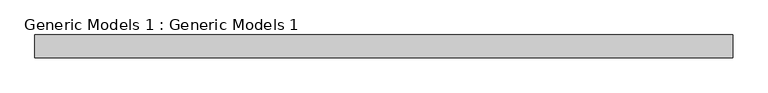
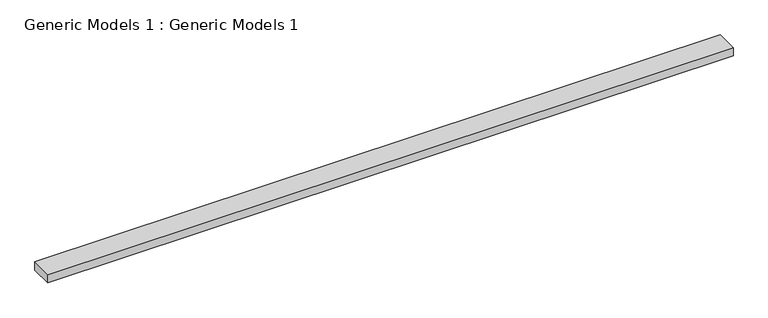
"""IFC4 building model written with IfcOpenShell, lengths in millimetres: proxy geometry, Generic Models 1 : Generic Models 1."""

from ifc_helpers import new_model, si_unit, frame, origin, place, context, project, spatial, polyline, outline, extrude, source, transform, mapped, element, save


def generic_models_1_generic_models_1_efd73d5e(model_context):
    return source(origin(), model_context, "Body", "SweptSolid", [
        extrude(outline(polyline([(12604.4370151, -3702.94432), (12604.4370151, -4404.8405988), (-8934.7629849, -4404.8405988), (-8934.7629849, -3702.94432), (12604.4370151, -3702.94432)])), frame((0.0, 0.0, 3139.6166481), z_axis=(0.0, 0.0, 1.0), x_axis=(1.0, 0.0, 0.0)), (0.0, 0.0, 1.0), 272.3536724),
    ])


if __name__ == "__main__":
    model = new_model("IFC4")
    model_context = context("Model", 3, world=origin())
    ifc_project = project(units=[si_unit("LENGTHUNIT", "METRE", prefix="MILLI")], contexts=[model_context])
    site = spatial("IfcSite", under=ifc_project)
    building = spatial("IfcBuilding", under=site)
    placement = place(None, origin())
    generic_models_1_generic_models_1_shape = generic_models_1_generic_models_1_efd73d5e(model_context)
    element("IfcBuildingElementProxy", 1, Name="Generic Models 1 : Generic Models 1", ObjectType="Generic Models 1 : Generic Models 1", at=placement, inside=building, context=model_context, shape_type="MappedRepresentation", body=[
        mapped(generic_models_1_generic_models_1_shape, transform((0.0, 0.0, 0.0), x_axis=(1.0, 0.0, 0.0), y_axis=(0.0, 1.0, 0.0), z_axis=(0.0, 0.0, 1.0))),
    ])
    save(model, "model.ifc")
